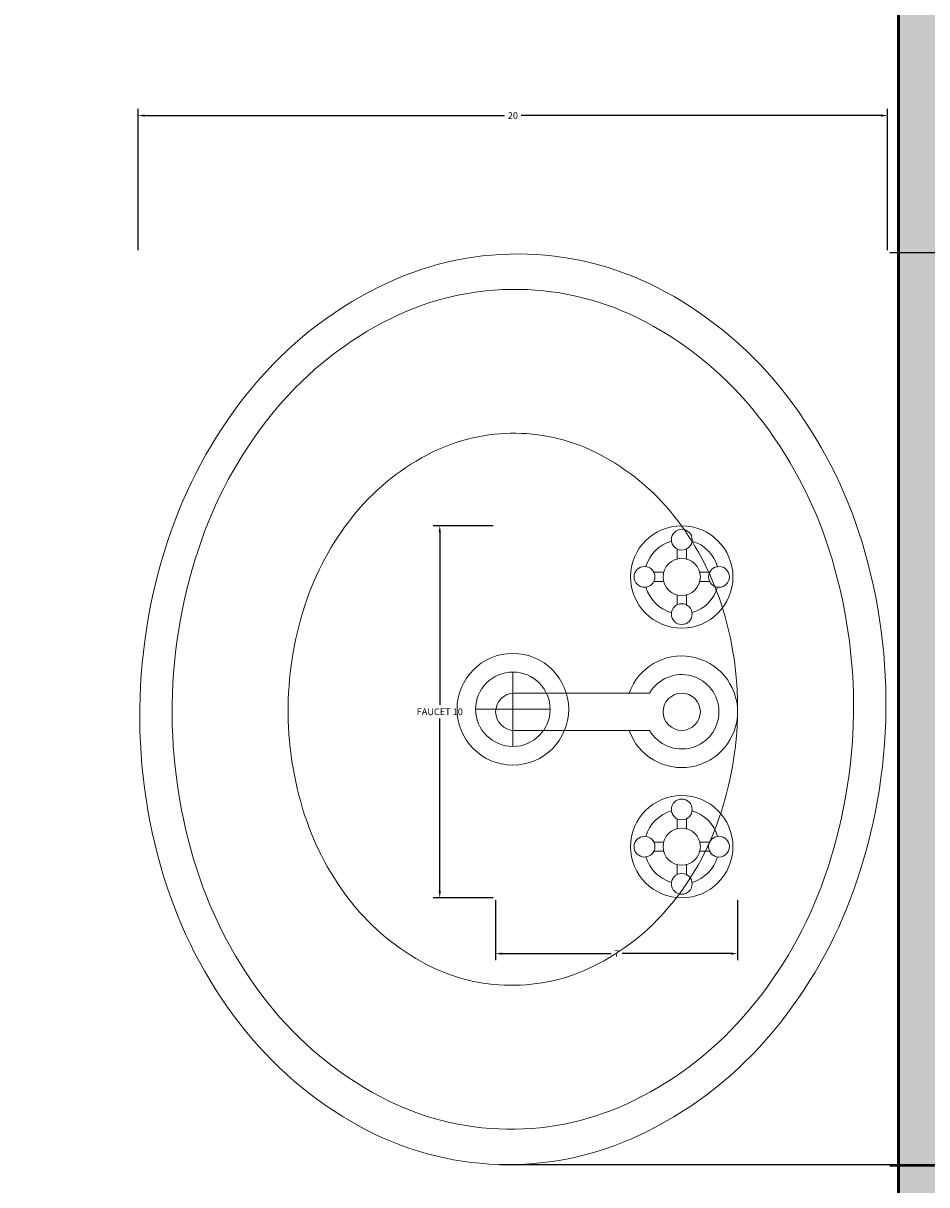
# Model space of a CAD drawing. Units: inches. Extents: x 2231 to 2461, y 2045 to 2455.
# Tile 84 of 95: x 2409 to 2434, y 2352 to 2383. Entities that reach past the tile are written whole.
import ezdxf

# ---------------------------------------------------------------- set-up
doc = ezdxf.new("R2010")
doc.units = ezdxf.units.IN
for name, color, linetype, lineweight in [('A-ANNO-DIMS', 2, 'Continuous', 18), ('A-FLOR-FIXT', 9, 'Continuous', 18), ('A-WALL', 7, 'Continuous', 50)]:
    doc.layers.add(name, color=color, linetype=linetype, lineweight=lineweight)
doc.layers.add('A-WALL-PATT', color=18, linetype='Continuous', lineweight=13, true_color=0x000000)
doc.styles.get("Standard").update_dxf_attribs({"font": 'arial.ttf'})
doc.dimstyles.get("Standard").update_dxf_attribs({"dimtxt": 0.18, "dimasz": 0.18, "dimexe": 0.18, "dimexo": 0.0625, "dimgap": 0.09, "dimtad": 0, "dimtih": 1, "dimtoh": 1, "dimdec": 4, "dimzin": 0, "dimdsep": 46, "dimtxsty": 'Standard', "dimcen": 0.09, "dimadec": 0, "dimazin": 0, "dimtfac": 1, "dimtdec": 4, "dimtofl": 0, "dimtmove": 0, "dimatfit": 3, "dimfxl": 1, "dimtolj": 1, "dimtzin": 0, "dimarcsym": 0})

# ---------------------------------------------------------------- blocks, each defined once
blk = doc.blocks.new('Sink - Oval top')
for p, q in [((0, 1), (0, -1)), ((-1, 0), (1, 0))]:
    blk.add_line(p, q)
for points in [[(-12.234, 0.394, 0.117634), (-11.465, -3.362, 0.104469), (-8.879, -6.804, 0.090016), (-5.083, -9.072, 0.08192), (-0.323, -10.016, 0.08192), (4.488, -9.381, 0.090016), (8.422, -7.361, 0.104469), (11.224, -4.093, 0.117634), (12.234, -0.394, 0.117634), (11.465, 3.362, 0.104469), (8.879, 6.804, 0.090016), (5.083, 9.072, 0.08192), (0.323, 10.016, 0.08192), (-4.488, 9.381, 0.090016), (-8.422, 7.361, 0.104469), (-11.224, 4.093, 0.117634)], [(-11.286, 0.159, 0.118622), (-10.516, -3.253, 0.104678), (-8.072, -6.359, 0.089562), (-4.538, -8.367, 0.081185), (-0.129, -9.152, 0.081185), (4.3, -8.492, 0.089562), (7.889, -6.584, 0.104678), (10.42, -3.548, 0.118622), (11.286, -0.159, 0.118622), (10.516, 3.253, 0.104678), (8.072, 6.359, 0.089562), (4.538, 8.367, 0.081185), (0.129, 9.152, 0.081185), (-4.3, 8.492, 0.089562), (-7.889, 6.584, 0.104678), (-10.42, 3.548, 0.118622)], [(-7.42, 0.083, 0.118283), (-6.907, -2.167, 0.104607), (-5.295, -4.21, 0.089718), (-2.967, -5.528, 0.081436), (-0.068, -6.037, 0.081436), (2.842, -5.593, 0.089718), (5.199, -4.327, 0.104607), (6.857, -2.321, 0.118283), (7.42, -0.083, 0.118283), (6.907, 2.167, 0.104607), (5.295, 4.21, 0.089718), (2.967, 5.528, 0.081436), (0.068, 6.037, 0.081436), (-2.842, 5.593, 0.089718), (-5.199, 4.327, 0.104607), (-6.857, 2.321, 0.118283)]]:
    blk.add_lwpolyline(points, format="xyb", close=True)
for radius in [1.5, 1]:
    blk.add_circle((0, 0), radius)
blk = doc.blocks.new('Faucet - Bathroom top')
for p, q in [((-3.75, 0.4788), (-3.75, 0.75)), ((-3.5, 0.482), (-3.5, 0.75)), ((3.5, 0.4788), (3.5, 0.75)), ((3.75, 0.482), (3.75, 0.75)), ((-4.107, 0.125), (-4.375, 0.125)), ((-3.1461, 0.125), (-2.875, 0.125)), ((3.143, 0.125), (2.875, 0.125)), ((4.1039, 0.125), (4.375, 0.125)), ((-4.1039, -0.125), (-4.375, -0.125)), ((-3.143, -0.125), (-2.875, -0.125)), ((3.1461, -0.125), (2.875, -0.125)), ((4.107, -0.125), (4.375, -0.125)), ((-3.75, -0.4821), (-3.75, -0.75)), ((-3.5, -0.4789), (-3.5, -0.75)), ((3.5, -0.4821), (3.5, -0.75)), ((3.75, -0.4789), (3.75, -0.75)), ((-0.5, -0.8639), (-0.5, -4.5)), ((0.5, -4.5), (0.5, -0.8631))]:
    blk.add_line(p, q)
for centre, radius in [((-3.625, 0), 1.375), ((-3.625, 1), 0.2795), ((3.625, 0), 1.375), ((3.625, 1), 0.2795), ((-3.625, 0), 0.5), ((0, 0), 0.5), ((3.625, 0), 0.5), ((-4.625, 0), 0.2795), ((-2.625, 0), 0.2795), ((2.625, 0), 0.2795), ((4.625, 0), 0.2795), ((-3.625, -1), 0.2795), ((3.625, -1), 0.2795)]:
    blk.add_circle(centre, radius)
for centre, radius, start, end in [((0, 0), 1.5, 289.6514, 250.3603), ((-3.625, 0), 1, 105.2407, 164.2093), ((-3.625, 0), 1, 16.44125, 74.07887), ((0, 0), 1, 300.3431, 239.7554), ((3.625, 0), 1, 106.12, 164.0884), ((3.625, 0), 1, 16.23422, 73.90469), ((-3.625, 0), 1, 196.2342, 253.9047), ((-3.625, 0), 1, 286.12, 344.0884), ((3.625, 0), 1, 196.4413, 254.0789), ((3.625, 0), 1, 285.2407, 344.2093), ((0, -4.5), 0.5, 180, 0)]:
    blk.add_arc(centre, radius, start, end)
blk = doc.blocks.new('*D23')
at = {"layer": 'A-ANNO-DIMS', "color": 0, "lineweight": -2, "transparency": 16777216}
for p, q in [((2432.568, 2377.172), (2436.368, 2377.172)), ((2436.188, 2376.992), (2436.188, 2365.08)), ((2436.188, 2352.802), (2436.188, 2364.714)), ((2432.568, 2352.622), (2436.368, 2352.622))]:
    blk.add_line(p, q, dxfattribs=at)
at = {"layer": 'A-ANNO-DIMS', "color": 0, "transparency": 16777216}
for points in [[(2436.158, 2376.992), (2436.218, 2376.992), (2436.188, 2377.172)], [(2436.158, 2352.802), (2436.218, 2352.802), (2436.188, 2352.622)]]:
    blk.add_solid(points, dxfattribs=at)
at = {"layer": 'Defpoints', "color": 0, "transparency": 16777216}
for p in [(2432.506, 2377.172), (2432.506, 2352.622), (2436.188, 2352.622)]:
    blk.add_point(p, dxfattribs=at)
at = {"layer": 'A-ANNO-DIMS', "color": 0, "transparency": 16777216, "insert": (2436.188, 2364.897), "char_height": 0.18, "attachment_point": 5}
blk.add_mtext('\\A1;BASIN 25', dxfattribs=at)
blk = doc.blocks.new('*D24')
at = {"layer": 'A-ANNO-DIMS', "color": 0, "lineweight": -2, "transparency": 16777216}
for p, q in [((2412.369, 2377.235), (2412.369, 2381.035)), ((2412.549, 2380.855), (2422.217, 2380.855)), ((2432.326, 2380.855), (2422.658, 2380.855)), ((2432.506, 2377.235), (2432.506, 2381.035))]:
    blk.add_line(p, q, dxfattribs=at)
at = {"layer": 'A-ANNO-DIMS', "color": 0, "transparency": 16777216}
for points in [[(2412.549, 2380.885), (2412.549, 2380.825), (2412.369, 2380.855)], [(2432.326, 2380.885), (2432.326, 2380.825), (2432.506, 2380.855)]]:
    blk.add_solid(points, dxfattribs=at)
at = {"layer": 'Defpoints', "color": 0, "transparency": 16777216}
for p in [(2432.506, 2380.855), (2412.369, 2377.172), (2432.506, 2377.172)]:
    blk.add_point(p, dxfattribs=at)
at = {"layer": 'A-ANNO-DIMS', "color": 0, "transparency": 16777216, "insert": (2422.438, 2380.855), "char_height": 0.18, "attachment_point": 5}
blk.add_mtext('\\A1;20', dxfattribs=at)
blk = doc.blocks.new('*D25')
at = {"layer": 'A-ANNO-DIMS', "color": 0, "lineweight": -2, "transparency": 16777216}
for p, q in [((2421.912, 2369.829), (2420.294, 2369.829)), ((2420.474, 2369.649), (2420.474, 2365.012)), ((2420.474, 2360.009), (2420.474, 2364.646)), ((2421.912, 2359.829), (2420.294, 2359.829))]:
    blk.add_line(p, q, dxfattribs=at)
at = {"layer": 'A-ANNO-DIMS', "color": 0, "transparency": 16777216}
for points in [[(2420.444, 2369.649), (2420.504, 2369.649), (2420.474, 2369.829)], [(2420.444, 2360.009), (2420.504, 2360.009), (2420.474, 2359.829)]]:
    blk.add_solid(points, dxfattribs=at)
at = {"layer": 'Defpoints', "color": 0, "transparency": 16777216}
for p in [(2421.974, 2369.829), (2420.474, 2359.829), (2421.974, 2359.829)]:
    blk.add_point(p, dxfattribs=at)
at = {"layer": 'A-ANNO-DIMS', "color": 0, "transparency": 16777216, "insert": (2420.474, 2364.829), "char_height": 0.18, "attachment_point": 5}
blk.add_mtext('\\A1;FAUCET 10', dxfattribs=at)
blk = doc.blocks.new('*D26')
at = {"layer": 'A-ANNO-DIMS', "color": 0, "lineweight": -2, "transparency": 16777216}
for p, q in [((2421.974, 2359.767), (2421.974, 2358.149)), ((2428.474, 2359.767), (2428.474, 2358.149)), ((2422.154, 2358.329), (2425.076, 2358.329)), ((2428.294, 2358.329), (2425.373, 2358.329))]:
    blk.add_line(p, q, dxfattribs=at)
at = {"layer": 'A-ANNO-DIMS', "color": 0, "transparency": 16777216}
for points in [[(2422.154, 2358.359), (2422.154, 2358.299), (2421.974, 2358.329)], [(2428.294, 2358.359), (2428.294, 2358.299), (2428.474, 2358.329)]]:
    blk.add_solid(points, dxfattribs=at)
at = {"layer": 'Defpoints', "color": 0, "transparency": 16777216}
for p in [(2421.974, 2359.829), (2428.474, 2359.829), (2428.474, 2358.329)]:
    blk.add_point(p, dxfattribs=at)
at = {"layer": 'A-ANNO-DIMS', "color": 0, "transparency": 16777216, "insert": (2425.224, 2358.329), "char_height": 0.18, "attachment_point": 5}
blk.add_mtext('\\A1;7', dxfattribs=at)
blk = doc.blocks.new('*D38')
at = {"layer": 'A-ANNO-DIMS', "color": 0, "lineweight": -2, "transparency": 16777216}
for p, q in [((2432.856, 2426.833), (2460.606, 2426.833)), ((2460.426, 2426.653), (2460.426, 2381.015)), ((2460.426, 2335.013), (2460.426, 2380.651)), ((2432.856, 2334.833), (2460.606, 2334.833))]:
    blk.add_line(p, q, dxfattribs=at)
at = {"layer": 'A-ANNO-DIMS', "color": 0, "transparency": 16777216}
for points in [[(2460.396, 2426.653), (2460.456, 2426.653), (2460.426, 2426.833)], [(2460.396, 2335.013), (2460.456, 2335.013), (2460.426, 2334.833)]]:
    blk.add_solid(points, dxfattribs=at)
at = {"layer": 'Defpoints', "color": 0, "transparency": 16777216}
for p in [(2432.794, 2426.833), (2460.426, 2426.833), (2432.794, 2334.833)]:
    blk.add_point(p, dxfattribs=at)
at = {"layer": 'A-ANNO-DIMS', "color": 0, "transparency": 16777216, "insert": (2460.426, 2380.833), "char_height": 0.18, "attachment_point": 5}
blk.add_mtext('\\A1;92', dxfattribs=at)
blk = doc.blocks.new('*D42')
at = {"layer": 'A-ANNO-DIMS', "color": 0, "lineweight": -2, "transparency": 16777216}
for p, q in [((2396.794, 2286.895), (2396.794, 2454.645)), ((2432.794, 2286.895), (2432.794, 2454.645)), ((2396.974, 2454.465), (2414.575, 2454.465)), ((2432.614, 2454.465), (2415.012, 2454.465))]:
    blk.add_line(p, q, dxfattribs=at)
at = {"layer": 'A-ANNO-DIMS', "color": 0, "transparency": 16777216}
for points in [[(2396.974, 2454.495), (2396.974, 2454.435), (2396.794, 2454.465)], [(2432.614, 2454.495), (2432.614, 2454.435), (2432.794, 2454.465)]]:
    blk.add_solid(points, dxfattribs=at)
at = {"layer": 'Defpoints', "color": 0, "transparency": 16777216}
for p in [(2432.794, 2454.465), (2396.794, 2286.833), (2432.794, 2286.833)]:
    blk.add_point(p, dxfattribs=at)
at = {"layer": 'A-ANNO-DIMS', "color": 0, "transparency": 16777216, "insert": (2414.794, 2454.465), "char_height": 0.18, "attachment_point": 5}
blk.add_mtext('\\A1;36', dxfattribs=at)
blk = doc.blocks.new('*D59')
at = {"layer": 'A-ANNO-DIMS', "color": 0, "lineweight": -2, "transparency": 16777216}
for p, q in [((2408.794, 2182.895), (2408.794, 2454.645)), ((2432.794, 2182.895), (2432.794, 2454.645)), ((2408.974, 2454.465), (2420.573, 2454.465)), ((2432.614, 2454.465), (2421.014, 2454.465))]:
    blk.add_line(p, q, dxfattribs=at)
at = {"layer": 'A-ANNO-DIMS', "color": 0, "transparency": 16777216}
for points in [[(2408.974, 2454.495), (2408.974, 2454.435), (2408.794, 2454.465)], [(2432.614, 2454.495), (2432.614, 2454.435), (2432.794, 2454.465)]]:
    blk.add_solid(points, dxfattribs=at)
at = {"layer": 'Defpoints', "color": 0, "transparency": 16777216}
for p in [(2432.794, 2454.465), (2408.794, 2182.833), (2432.794, 2182.833)]:
    blk.add_point(p, dxfattribs=at)
at = {"layer": 'A-ANNO-DIMS', "color": 0, "transparency": 16777216, "insert": (2420.794, 2454.465), "char_height": 0.18, "attachment_point": 5}
blk.add_mtext('\\A1;24', dxfattribs=at)
blk = doc.blocks.new('*D76')
at = {"layer": 'A-ANNO-DIMS', "color": 0, "lineweight": -2, "transparency": 16777216}
for p, q in [((2422.106, 2352.663), (2460.606, 2352.663)), ((2460.426, 2352.483), (2460.426, 2343.93)), ((2460.426, 2335.013), (2460.426, 2343.566)), ((2432.856, 2334.833), (2460.606, 2334.833))]:
    blk.add_line(p, q, dxfattribs=at)
at = {"layer": 'A-ANNO-DIMS', "color": 0, "transparency": 16777216}
for points in [[(2460.396, 2352.483), (2460.456, 2352.483), (2460.426, 2352.663)], [(2460.396, 2335.013), (2460.456, 2335.013), (2460.426, 2334.833)]]:
    blk.add_solid(points, dxfattribs=at)
at = {"layer": 'Defpoints', "color": 0, "transparency": 16777216}
for p in [(2422.043, 2352.663), (2460.426, 2352.663), (2432.794, 2334.833)]:
    blk.add_point(p, dxfattribs=at)
at = {"layer": 'A-ANNO-DIMS', "color": 0, "transparency": 16777216, "insert": (2460.426, 2343.748), "char_height": 0.18, "attachment_point": 5}
blk.add_mtext('\\A1;17.83', dxfattribs=at)

msp = doc.modelspace()

# ---------------------------------------------------------------- hatches: boundary and pattern name
at = {"layer": 'A-WALL-PATT'}
h = msp.add_hatch(color=256, dxfattribs=at)
h.dxf.hatch_style = 1
h.paths.add_polyline_path([(2441.7935, 2269.1535), (2432.7935, 2269.1535), (2432.7935, 2186.8328), (2396.7935, 2186.8328), (2396.7935, 2286.8328), (2394.7935, 2286.8328), (2394.7935, 2186.8328), (2334.7935, 2186.8328), (2334.7935, 2182.8328), (2432.7935, 2182.8328), (2432.7935, 2072.8328), (2416.6639, 2072.8328), (2416.6639, 2063.8328), (2441.7935, 2063.8328)])
h.paths.add_polyline_path([(2368.6639, 2072.8328), (2367.04, 2072.8328), (2330.7942, 2072.8328), (2330.7397, 2063.8328), (2368.6639, 2063.8328)])
h.paths.add_polyline_path([(2300.7392, 2068.3328), (2300.7392, 2072.8328), (2298.7935, 2072.8328), (2294.7935, 2072.8328), (2258.7935, 2072.8328), (2258.7935, 2120.8328), (2294.7935, 2120.8328), (2298.7935, 2120.8328), (2298.7935, 2128.8328), (2294.7935, 2128.8328), (2294.7935, 2124.8328), (2258.7935, 2124.8328), (2258.7935, 2182.8328), (2294.7935, 2182.8328), (2294.7935, 2174.8328), (2298.7935, 2174.8328), (2298.7935, 2182.8328), (2304.7935, 2182.8328), (2304.7935, 2186.8328), (2258.7935, 2186.8328), (2258.7935, 2221.999), (2249.7935, 2221.999), (2249.7935, 2063.8328), (2300.7392, 2063.8328)])
h.paths.add_polyline_path([(2391.9338, 2435.8328), (2333.82, 2435.8328), (2333.82, 2426.8328), (2368.7935, 2426.8328), (2368.7935, 2374.9508), (2368.7935, 2370.8328), (2372.3935, 2370.8328), (2372.7935, 2370.8328), (2372.7935, 2426.8328), (2391.9338, 2426.8328)])
h.paths.add_polyline_path([(2441.7935, 2435.8328), (2415.9338, 2435.8328), (2415.9338, 2426.8328), (2432.7935, 2426.8328), (2432.7935, 2334.8328), (2372.7935, 2334.8328), (2372.7935, 2346.8328), (2368.7935, 2346.8328), (2368.7935, 2306.8328), (2360.7935, 2306.8328), (2360.7935, 2302.8328), (2368.7935, 2302.8328), (2372.7935, 2302.8328), (2372.7935, 2330.8328), (2432.7935, 2330.8328), (2432.7935, 2317.1535), (2441.7935, 2317.1535)])
h.paths.add_polyline_path([(2285.82, 2435.8328), (2249.7935, 2435.8328), (2249.7935, 2269.999), (2258.7935, 2269.999), (2258.7935, 2302.8328), (2318.8168, 2302.8328), (2330.7935, 2302.8328), (2330.7935, 2306.8328), (2258.7935, 2306.8328), (2258.7935, 2426.8328), (2285.82, 2426.8328)])

# ---------------------------------------------------------------- linework, layer by layer
at = {"layer": 'A-WALL'}
msp.add_line((2432.7935, 2426.8328), (2432.7935, 2334.8328), dxfattribs=at)

# ---------------------------------------------------------------- block references
at = {"layer": 'A-FLOR-FIXT', "rotation": 270}
for name, p in [('Sink - Oval top', (2422.4375, 2364.897)), ('Faucet - Bathroom top', (2426.9743, 2364.8294))]:
    msp.add_blockref(name, p, dxfattribs=at)

# ---------------------------------------------------------------- dimensions: what is measured, and where the dimension line sits
at = {"layer": 'A-ANNO-DIMS'}
for base, p1, p2, picture, middle in [((2432.7935, 2454.4653), (2396.7935, 2286.8328), (2432.7935, 2286.8328), '*D42', (2414.7935, 2454.4653)), ((2432.7935, 2454.4653), (2408.7935, 2182.8328), (2432.7935, 2182.8328), '*D59', (2420.7935, 2454.4653)), ((2432.5058, 2380.8551), (2412.3692, 2377.1725), (2432.5058, 2377.1725), '*D24', (2422.4375, 2380.8551)), ((2428.4744, 2358.3294), (2421.9743, 2359.8294), (2428.4744, 2359.8294), '*D26', (2425.2244, 2358.3294))]:
    dim = msp.add_linear_dim(base=base, p1=p1, p2=p2, dimstyle='Standard', override={"dimdec": 0, "dimlfac": 1, "dimrnd": 0, "dimzin": 0, "dimdsep": 46, "dimlunit": 2}, dxfattribs=at)
    dim.commit()
    dim.dimension.update_dxf_attribs({"geometry": picture, "text_midpoint": middle})
for base, p2, override, picture, middle in [((2460.426, 2426.8328), (2432.7935, 2426.8328), {"dimdec": 0, "dimlfac": 1, "dimrnd": 0, "dimzin": 0, "dimdsep": 46, "dimlunit": 2}, '*D38', (2460.426, 2380.8328)), ((2460.426, 2352.6633), (2422.0433, 2352.6633), {"dimdec": 2, "dimlfac": 1, "dimrnd": 0, "dimzin": 0, "dimdsep": 46, "dimlunit": 2}, '*D76', (2460.426, 2343.7481))]:
    dim = msp.add_linear_dim(base=base, p1=(2432.7935, 2334.8328), p2=p2, angle=90, dimstyle='Standard', override=override, dxfattribs=at)
    dim.commit()
    dim.dimension.update_dxf_attribs({"geometry": picture, "text_midpoint": middle})
for base, p1, p2, text, picture, middle in [((2436.1885, 2352.6216), (2432.5058, 2377.1725), (2432.5058, 2352.6216), 'BASIN <>', '*D23', (2436.1885, 2364.897)), ((2420.4743, 2359.8294), (2421.9743, 2369.8294), (2421.9743, 2359.8294), 'FAUCET <>', '*D25', (2420.4743, 2364.8294))]:
    dim = msp.add_linear_dim(base=base, p1=p1, p2=p2, angle=270, text=text, dimstyle='Standard', override={"dimdec": 0, "dimlfac": 1, "dimrnd": 0, "dimzin": 0, "dimdsep": 46, "dimlunit": 2}, dxfattribs=at)
    dim.commit()
    dim.dimension.update_dxf_attribs({"geometry": picture, "text_midpoint": middle})

doc.saveas('drawing.dxf')
